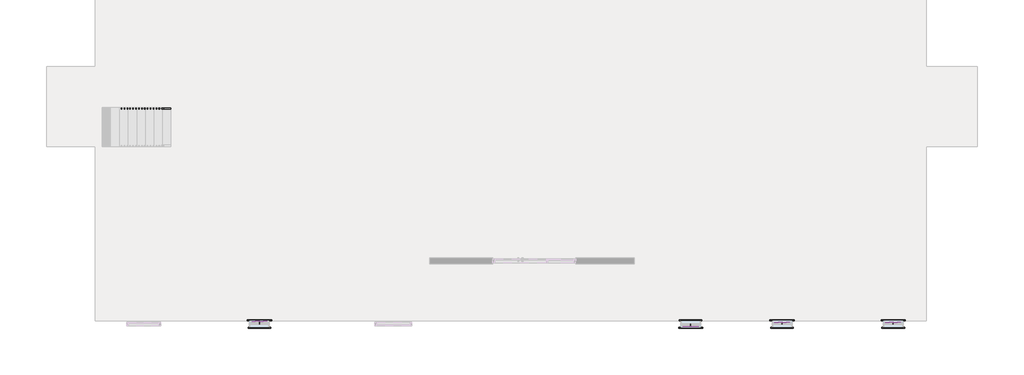
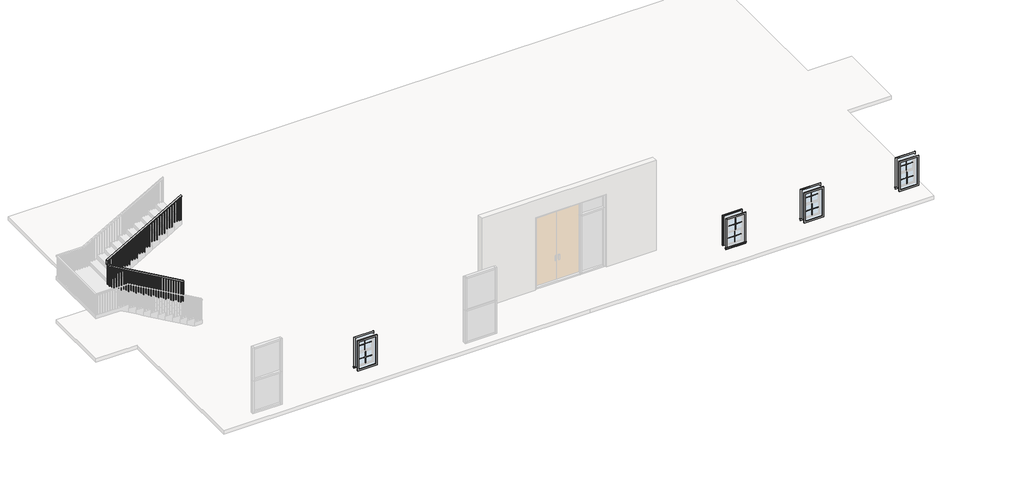
# One storey, part 3 of 3: 16 proxies, 1 railing.
"""IFC4 building model written with IfcOpenShell, lengths in millimetres."""

from ifc_helpers import new_model, si_unit, frame, origin, place, context, project, spatial, polyline, outline, extrude, faceted_brep, transform, mapped, element, save
from components import m_muntin_pattern_2x2_m_muntin_pattern_2x2_8c828626, m_trim_window_exterior_flat_with_sill_7a42a2ef, m_trim_window_interior_flat_picture_frame_c294611c

model = new_model("IFC4")

# Units and contexts
model_context = context("Model", 3, world=origin())
ifc_project = project(units=[si_unit("LENGTHUNIT", "METRE", prefix="MILLI")], contexts=[model_context])

# Site, building, storey
site = spatial("IfcSite", under=ifc_project)
building = spatial("IfcBuilding", under=site)
storey = spatial("IfcBuildingStorey", under=building, Elevation=600.0)

# Proxies
placement = place(None, origin())
m_muntin_pattern_2x2_m_muntin_pattern_2x2_shape = m_muntin_pattern_2x2_m_muntin_pattern_2x2_8c828626(model_context)
element("IfcBuildingElementProxy", 1, Name="M_Muntin Pattern_2x2 : M_Muntin Pattern_2x2", ObjectType="M_Muntin Pattern_2x2 : M_Muntin Pattern_2x2", at=placement, inside=storey, context=model_context, shape_type="MappedRepresentation", body=[
    mapped(m_muntin_pattern_2x2_m_muntin_pattern_2x2_shape, transform((11343.5830368, -12943.1342374, 2136.625), x_axis=(-1.0, 0.0, 0.0), y_axis=(0.0, -1.0, 0.0), z_axis=(0.0, 0.0, 1.0))),
])
element("IfcBuildingElementProxy", 2, Name="M_Muntin Pattern_2x2 : M_Muntin Pattern_2x2", ObjectType="M_Muntin Pattern_2x2 : M_Muntin Pattern_2x2", at=placement, inside=storey, context=model_context, shape_type="MappedRepresentation", body=[
    mapped(m_muntin_pattern_2x2_m_muntin_pattern_2x2_shape, transform((11343.5830368, -12898.6842374, 1590.6), x_axis=(-1.0, 0.0, 0.0), y_axis=(0.0, -1.0, 0.0), z_axis=(0.0, 0.0, 1.0))),
])
element("IfcBuildingElementProxy", 3, Name="M_Muntin Pattern_2x2 : M_Muntin Pattern_2x2", ObjectType="M_Muntin Pattern_2x2 : M_Muntin Pattern_2x2", at=placement, inside=storey, context=model_context, shape_type="MappedRepresentation", body=[
    mapped(m_muntin_pattern_2x2_m_muntin_pattern_2x2_shape, transform((14543.5830368, -12787.9842374, 2136.625), x_axis=(1.0, 0.0, 0.0), y_axis=(0.0, 1.0, 0.0), z_axis=(0.0, 0.0, 1.0))),
])
element("IfcBuildingElementProxy", 4, Name="M_Muntin Pattern_2x2 : M_Muntin Pattern_2x2", ObjectType="M_Muntin Pattern_2x2 : M_Muntin Pattern_2x2", at=placement, inside=storey, context=model_context, shape_type="MappedRepresentation", body=[
    mapped(m_muntin_pattern_2x2_m_muntin_pattern_2x2_shape, transform((14543.5830368, -12832.4342374, 1590.6), x_axis=(1.0, 0.0, 0.0), y_axis=(0.0, 1.0, 0.0), z_axis=(0.0, 0.0, 1.0))),
])
element("IfcBuildingElementProxy", 5, Name="M_Muntin Pattern_2x2 : M_Muntin Pattern_2x2", ObjectType="M_Muntin Pattern_2x2 : M_Muntin Pattern_2x2", at=placement, inside=storey, context=model_context, shape_type="MappedRepresentation", body=[
    mapped(m_muntin_pattern_2x2_m_muntin_pattern_2x2_shape, transform((18431.0830368, -12787.9842374, 2136.625), x_axis=(1.0, 0.0, 0.0), y_axis=(0.0, 1.0, 0.0), z_axis=(0.0, 0.0, 1.0))),
])
element("IfcBuildingElementProxy", 6, Name="M_Muntin Pattern_2x2 : M_Muntin Pattern_2x2", ObjectType="M_Muntin Pattern_2x2 : M_Muntin Pattern_2x2", at=placement, inside=storey, context=model_context, shape_type="MappedRepresentation", body=[
    mapped(m_muntin_pattern_2x2_m_muntin_pattern_2x2_shape, transform((18431.0830368, -12832.4342374, 1590.6), x_axis=(1.0, 0.0, 0.0), y_axis=(0.0, 1.0, 0.0), z_axis=(0.0, 0.0, 1.0))),
])
element("IfcBuildingElementProxy", 7, Name="M_Muntin Pattern_2x2 : M_Muntin Pattern_2x2", ObjectType="M_Muntin Pattern_2x2 : M_Muntin Pattern_2x2", at=placement, inside=storey, context=model_context, shape_type="MappedRepresentation", body=[
    mapped(m_muntin_pattern_2x2_m_muntin_pattern_2x2_shape, transform((-3743.9169632, -12787.9842374, 2136.625), x_axis=(1.0, 0.0, 0.0), y_axis=(0.0, 1.0, 0.0), z_axis=(0.0, 0.0, 1.0))),
])
element("IfcBuildingElementProxy", 8, Name="M_Muntin Pattern_2x2 : M_Muntin Pattern_2x2", ObjectType="M_Muntin Pattern_2x2 : M_Muntin Pattern_2x2", at=placement, inside=storey, context=model_context, shape_type="MappedRepresentation", body=[
    mapped(m_muntin_pattern_2x2_m_muntin_pattern_2x2_shape, transform((-3743.9169632, -12832.4342374, 1590.6), x_axis=(1.0, 0.0, 0.0), y_axis=(0.0, 1.0, 0.0), z_axis=(0.0, 0.0, 1.0))),
])
m_trim_window_exterior_flat_with_sill_shape = m_trim_window_exterior_flat_with_sill_7a42a2ef(model_context)
element("IfcBuildingElementProxy", 9, Name="M_Trim-Window-Exterior-Flat : with Sill", ObjectType="M_Trim-Window-Exterior-Flat : with Sill", at=placement, inside=storey, context=model_context, shape_type="MappedRepresentation", body=[
    mapped(m_trim_window_exterior_flat_with_sill_shape, transform((11343.5830368, -12978.0592374, 2714.4), x_axis=(1.0, 0.0, 0.0), y_axis=(0.0, 0.0, 1.0), z_axis=(0.0, -1.0, 0.0))),
])
element("IfcBuildingElementProxy", 10, Name="M_Trim-Window-Exterior-Flat : with Sill", ObjectType="M_Trim-Window-Exterior-Flat : with Sill", at=placement, inside=storey, context=model_context, shape_type="MappedRepresentation", body=[
    mapped(m_trim_window_exterior_flat_with_sill_shape, transform((14543.5830368, -12753.0592374, 2714.4), x_axis=(-1.0, 0.0, 0.0), y_axis=(0.0, 0.0, 1.0), z_axis=(0.0, 1.0, 0.0))),
])
element("IfcBuildingElementProxy", 11, Name="M_Trim-Window-Exterior-Flat : with Sill", ObjectType="M_Trim-Window-Exterior-Flat : with Sill", at=placement, inside=storey, context=model_context, shape_type="MappedRepresentation", body=[
    mapped(m_trim_window_exterior_flat_with_sill_shape, transform((18431.0830368, -12753.0592374, 2714.4), x_axis=(-1.0, 0.0, 0.0), y_axis=(0.0, 0.0, 1.0), z_axis=(0.0, 1.0, 0.0))),
])
element("IfcBuildingElementProxy", 12, Name="M_Trim-Window-Exterior-Flat : with Sill", ObjectType="M_Trim-Window-Exterior-Flat : with Sill", at=placement, inside=storey, context=model_context, shape_type="MappedRepresentation", body=[
    mapped(m_trim_window_exterior_flat_with_sill_shape, transform((-3743.9169632, -12753.0592374, 2714.4), x_axis=(-1.0, 0.0, 0.0), y_axis=(0.0, 0.0, 1.0), z_axis=(0.0, 1.0, 0.0))),
])
m_trim_window_interior_flat_picture_frame_shape = m_trim_window_interior_flat_picture_frame_c294611c(model_context)
element("IfcBuildingElementProxy", 13, Name="M_Trim-Window-Interior-Flat : Picture Frame", ObjectType="M_Trim-Window-Interior-Flat : Picture Frame", at=placement, inside=storey, context=model_context, shape_type="MappedRepresentation", body=[
    mapped(m_trim_window_interior_flat_picture_frame_shape, transform((11343.5830368, -12753.0592374, 2714.4), x_axis=(-1.0, 0.0, 0.0), y_axis=(0.0, 0.0, 1.0), z_axis=(0.0, 1.0, 0.0))),
])
element("IfcBuildingElementProxy", 14, Name="M_Trim-Window-Interior-Flat : Picture Frame", ObjectType="M_Trim-Window-Interior-Flat : Picture Frame", at=placement, inside=storey, context=model_context, shape_type="MappedRepresentation", body=[
    mapped(m_trim_window_interior_flat_picture_frame_shape, transform((14543.5830368, -12978.0592374, 2714.4), x_axis=(1.0, 0.0, 0.0), y_axis=(0.0, 0.0, 1.0), z_axis=(0.0, -1.0, 0.0))),
])
element("IfcBuildingElementProxy", 15, Name="M_Trim-Window-Interior-Flat : Picture Frame", ObjectType="M_Trim-Window-Interior-Flat : Picture Frame", at=placement, inside=storey, context=model_context, shape_type="MappedRepresentation", body=[
    mapped(m_trim_window_interior_flat_picture_frame_shape, transform((18431.0830368, -12978.0592374, 2714.4), x_axis=(1.0, 0.0, 0.0), y_axis=(0.0, 0.0, 1.0), z_axis=(0.0, -1.0, 0.0))),
])
element("IfcBuildingElementProxy", 16, Name="M_Trim-Window-Interior-Flat : Picture Frame", ObjectType="M_Trim-Window-Interior-Flat : Picture Frame", at=placement, inside=storey, context=model_context, shape_type="MappedRepresentation", body=[
    mapped(m_trim_window_interior_flat_picture_frame_shape, transform((-3743.9169632, -12978.0592374, 2714.4), x_axis=(1.0, 0.0, 0.0), y_axis=(0.0, 0.0, 1.0), z_axis=(0.0, -1.0, 0.0))),
])

# Railing
element("IfcRailing", 17, ObjectType="Handrail - Rectangular", at=placement, inside=storey, context=model_context, shape_type="SolidModel", body=[
    faceted_brep([(-6843.9169632, -5340.9592374, 1671.4285714), (-6843.9169632, -5340.9592374, 1613.8410161), (-6843.9169632, -5290.9592374, 1613.8410161), (-6843.9169632, -5290.9592374, 1671.4285714), (-9769.3169632, -5340.9592374, 3343.0857143), (-9819.3169632, -5340.9592374, 3314.0695875), (-9819.3169632, -5290.9592374, 3314.0695875), (-9769.3169632, -5290.9592374, 3343.0857143), (-9769.3169632, -5340.9592374, 3385.7142857), (-9819.3169632, -5340.9592374, 3335.7142857), (-9819.3169632, -5290.9592374, 3335.7142857), (-9769.3169632, -5290.9592374, 3385.7142857), (-9894.3169632, -5340.9592374, 3385.7142857), (-9894.3169632, -5340.9592374, 3335.7142857), (-9844.3169632, -5290.9592374, 3335.7142857), (-9844.3169632, -5290.9592374, 3385.7142857), (-9894.3169632, -5215.9592374, 3385.7142857), (-9894.3169632, -5215.9592374, 3335.7142857), (-9844.3169632, -5215.9592374, 3335.7142857), (-9844.3169632, -5215.9592374, 3385.7142857), (-9894.3169632, -5190.1592374, 3385.7142857), (-9844.3169632, -5190.1592374, 3385.7142857), (-9844.3169632, -5140.1592374, 3335.7142857), (-9894.3169632, -5140.1592374, 3335.7142857)], [[[0, 1, 2, 3]], [[1, 0, 4, 5]], [[2, 1, 5, 6]], [[3, 2, 6, 7]], [[0, 3, 7, 4]], [[5, 4, 8, 9]], [[6, 5, 9, 10]], [[7, 6, 10, 11]], [[4, 7, 11, 8]], [[9, 8, 12, 13]], [[10, 9, 13, 14]], [[11, 10, 14, 15]], [[8, 11, 15, 12]], [[13, 12, 16, 17]], [[14, 13, 17, 18]], [[15, 14, 18, 19]], [[12, 15, 19, 16]], [[20, 21, 22, 23]], [[17, 16, 20, 23]], [[18, 17, 23, 22]], [[19, 18, 22, 21]], [[16, 19, 21, 20]]]),
    faceted_brep([(-9894.3169632, -5190.1592374, 3385.7142857), (-9894.3169632, -5140.1592374, 3335.7142857), (-9844.3169632, -5140.1592374, 3335.7142857), (-9844.3169632, -5190.1592374, 3385.7142857), (-9894.3169632, -5190.1592374, 3528.3428571), (-9844.3169632, -5190.1592374, 3499.3267304), (-9844.3169632, -5140.1592374, 3499.3267304), (-9894.3169632, -5140.1592374, 3528.3428571)], [[[0, 1, 2, 3]], [[4, 5, 6, 7]], [[1, 0, 4, 7]], [[2, 1, 7, 6]], [[3, 2, 6, 5]], [[0, 3, 5, 4]]]),
    faceted_brep([(-9894.3169632, -5140.1592374, 3528.3428571), (-9844.3169632, -5140.1592374, 3499.3267304), (-9844.3169632, -5190.1592374, 3499.3267304), (-9894.3169632, -5190.1592374, 3528.3428571), (-6843.9169632, -5140.1592374, 5271.4285714), (-6843.9169632, -5190.1592374, 5271.4285714), (-6843.9169632, -5190.1592374, 5213.8410161), (-6843.9169632, -5140.1592374, 5213.8410161)], [[[0, 1, 2, 3]], [[4, 5, 6, 7]], [[1, 0, 4, 7]], [[2, 1, 7, 6]], [[3, 2, 6, 5]], [[0, 3, 5, 4]]]),
    extrude(outline(polyline([(5162.9838732, -6932.9169632), (4200.0, -6932.9169632), (4200.0, -6912.9169632), (5174.4124447, -6912.9169632), (5162.9838732, -6932.9169632)])), frame((0.0, -5175.1592374, 0.0), z_axis=(0.0, 1.0, 0.0), x_axis=(0.0, 0.0, 1.0)), (0.0, 0.0, 1.0), 20.0),
    extrude(outline(polyline([(5104.9267304, -7034.5169632), (4200.0, -7034.5169632), (4200.0, -7014.5169632), (5116.3553018, -7014.5169632), (5104.9267304, -7034.5169632)])), frame((0.0, -5175.1592374, 0.0), z_axis=(0.0, 1.0, 0.0), x_axis=(0.0, 0.0, 1.0)), (0.0, 0.0, 1.0), 20.0),
    extrude(outline(polyline([(5046.8695875, -7136.1169632), (4200.0, -7136.1169632), (4200.0, -7116.1169632), (5058.2981589, -7116.1169632), (5046.8695875, -7136.1169632)])), frame((0.0, -5175.1592374, 0.0), z_axis=(0.0, 1.0, 0.0), x_axis=(0.0, 0.0, 1.0)), (0.0, 0.0, 1.0), 20.0),
    extrude(outline(polyline([(4988.8124447, -7237.7169632), (4028.5714286, -7237.7169632), (4028.5714286, -7217.7169632), (5000.2410161, -7217.7169632), (4988.8124447, -7237.7169632)])), frame((0.0, -5175.1592374, 0.0), z_axis=(0.0, 1.0, 0.0), x_axis=(0.0, 0.0, 1.0)), (0.0, 0.0, 1.0), 20.0),
    extrude(outline(polyline([(4930.7553018, -7339.3169632), (4028.5714286, -7339.3169632), (4028.5714286, -7319.3169632), (4942.1838732, -7319.3169632), (4930.7553018, -7339.3169632)])), frame((0.0, -5175.1592374, 0.0), z_axis=(0.0, 1.0, 0.0), x_axis=(0.0, 0.0, 1.0)), (0.0, 0.0, 1.0), 20.0),
    extrude(outline(polyline([(4872.6981589, -7440.9169632), (4028.5714286, -7440.9169632), (4028.5714286, -7420.9169632), (4884.1267304, -7420.9169632), (4872.6981589, -7440.9169632)])), frame((0.0, -5175.1592374, 0.0), z_axis=(0.0, 1.0, 0.0), x_axis=(0.0, 0.0, 1.0)), (0.0, 0.0, 1.0), 20.0),
    extrude(outline(polyline([(4814.6410161, -7542.5169632), (3857.1428571, -7542.5169632), (3857.1428571, -7522.5169632), (4826.0695875, -7522.5169632), (4814.6410161, -7542.5169632)])), frame((0.0, -5175.1592374, 0.0), z_axis=(0.0, 1.0, 0.0), x_axis=(0.0, 0.0, 1.0)), (0.0, 0.0, 1.0), 20.0),
    extrude(outline(polyline([(4756.5838732, -7644.1169632), (3857.1428571, -7644.1169632), (3857.1428571, -7624.1169632), (4768.0124447, -7624.1169632), (4756.5838732, -7644.1169632)])), frame((0.0, -5175.1592374, 0.0), z_axis=(0.0, 1.0, 0.0), x_axis=(0.0, 0.0, 1.0)), (0.0, 0.0, 1.0), 20.0),
    extrude(outline(polyline([(4698.5267304, -7745.7169632), (3857.1428571, -7745.7169632), (3857.1428571, -7725.7169632), (4709.9553018, -7725.7169632), (4698.5267304, -7745.7169632)])), frame((0.0, -5175.1592374, 0.0), z_axis=(0.0, 1.0, 0.0), x_axis=(0.0, 0.0, 1.0)), (0.0, 0.0, 1.0), 20.0),
    extrude(outline(polyline([(4640.4695875, -7847.3169632), (3685.7142857, -7847.3169632), (3685.7142857, -7827.3169632), (4651.8981589, -7827.3169632), (4640.4695875, -7847.3169632)])), frame((0.0, -5175.1592374, 0.0), z_axis=(0.0, 1.0, 0.0), x_axis=(0.0, 0.0, 1.0)), (0.0, 0.0, 1.0), 20.0),
    extrude(outline(polyline([(4582.4124447, -7948.9169632), (3685.7142857, -7948.9169632), (3685.7142857, -7928.9169632), (4593.8410161, -7928.9169632), (4582.4124447, -7948.9169632)])), frame((0.0, -5175.1592374, 0.0), z_axis=(0.0, 1.0, 0.0), x_axis=(0.0, 0.0, 1.0)), (0.0, 0.0, 1.0), 20.0),
    extrude(outline(polyline([(4524.3553018, -8050.5169632), (3685.7142857, -8050.5169632), (3685.7142857, -8030.5169632), (4535.7838732, -8030.5169632), (4524.3553018, -8050.5169632)])), frame((0.0, -5175.1592374, 0.0), z_axis=(0.0, 1.0, 0.0), x_axis=(0.0, 0.0, 1.0)), (0.0, 0.0, 1.0), 20.0),
    extrude(outline(polyline([(4466.2981589, -8152.1169632), (3514.2857143, -8152.1169632), (3514.2857143, -8132.1169632), (4477.7267304, -8132.1169632), (4466.2981589, -8152.1169632)])), frame((0.0, -5175.1592374, 0.0), z_axis=(0.0, 1.0, 0.0), x_axis=(0.0, 0.0, 1.0)), (0.0, 0.0, 1.0), 20.0),
    extrude(outline(polyline([(4408.2410161, -8253.7169632), (3514.2857143, -8253.7169632), (3514.2857143, -8233.7169632), (4419.6695875, -8233.7169632), (4408.2410161, -8253.7169632)])), frame((0.0, -5175.1592374, 0.0), z_axis=(0.0, 1.0, 0.0), x_axis=(0.0, 0.0, 1.0)), (0.0, 0.0, 1.0), 20.0),
    extrude(outline(polyline([(4350.1838732, -8355.3169632), (3342.8571429, -8355.3169632), (3342.8571429, -8335.3169632), (4361.6124447, -8335.3169632), (4350.1838732, -8355.3169632)])), frame((0.0, -5175.1592374, 0.0), z_axis=(0.0, 1.0, 0.0), x_axis=(0.0, 0.0, 1.0)), (0.0, 0.0, 1.0), 20.0),
    extrude(outline(polyline([(4292.1267304, -8456.9169632), (3342.8571429, -8456.9169632), (3342.8571429, -8436.9169632), (4303.5553018, -8436.9169632), (4292.1267304, -8456.9169632)])), frame((0.0, -5175.1592374, 0.0), z_axis=(0.0, 1.0, 0.0), x_axis=(0.0, 0.0, 1.0)), (0.0, 0.0, 1.0), 20.0),
    extrude(outline(polyline([(4234.0695875, -8558.5169632), (3342.8571429, -8558.5169632), (3342.8571429, -8538.5169632), (4245.4981589, -8538.5169632), (4234.0695875, -8558.5169632)])), frame((0.0, -5175.1592374, 0.0), z_axis=(0.0, 1.0, 0.0), x_axis=(0.0, 0.0, 1.0)), (0.0, 0.0, 1.0), 20.0),
    extrude(outline(polyline([(4176.0124447, -8660.1169632), (3171.4285714, -8660.1169632), (3171.4285714, -8640.1169632), (4187.4410161, -8640.1169632), (4176.0124447, -8660.1169632)])), frame((0.0, -5175.1592374, 0.0), z_axis=(0.0, 1.0, 0.0), x_axis=(0.0, 0.0, 1.0)), (0.0, 0.0, 1.0), 20.0),
    extrude(outline(polyline([(4117.9553018, -8761.7169632), (3171.4285714, -8761.7169632), (3171.4285714, -8741.7169632), (4129.3838732, -8741.7169632), (4117.9553018, -8761.7169632)])), frame((0.0, -5175.1592374, 0.0), z_axis=(0.0, 1.0, 0.0), x_axis=(0.0, 0.0, 1.0)), (0.0, 0.0, 1.0), 20.0),
    extrude(outline(polyline([(4059.8981589, -8863.3169632), (3171.4285714, -8863.3169632), (3171.4285714, -8843.3169632), (4071.3267304, -8843.3169632), (4059.8981589, -8863.3169632)])), frame((0.0, -5175.1592374, 0.0), z_axis=(0.0, 1.0, 0.0), x_axis=(0.0, 0.0, 1.0)), (0.0, 0.0, 1.0), 20.0),
    extrude(outline(polyline([(4001.8410161, -8964.9169632), (3000.0, -8964.9169632), (3000.0, -8944.9169632), (4013.2695875, -8944.9169632), (4001.8410161, -8964.9169632)])), frame((0.0, -5175.1592374, 0.0), z_axis=(0.0, 1.0, 0.0), x_axis=(0.0, 0.0, 1.0)), (0.0, 0.0, 1.0), 20.0),
    extrude(outline(polyline([(3943.7838732, -9066.5169632), (3000.0, -9066.5169632), (3000.0, -9046.5169632), (3955.2124447, -9046.5169632), (3943.7838732, -9066.5169632)])), frame((0.0, -5175.1592374, 0.0), z_axis=(0.0, 1.0, 0.0), x_axis=(0.0, 0.0, 1.0)), (0.0, 0.0, 1.0), 20.0),
    extrude(outline(polyline([(3885.7267304, -9168.1169632), (3000.0, -9168.1169632), (3000.0, -9148.1169632), (3897.1553018, -9148.1169632), (3885.7267304, -9168.1169632)])), frame((0.0, -5175.1592374, 0.0), z_axis=(0.0, 1.0, 0.0), x_axis=(0.0, 0.0, 1.0)), (0.0, 0.0, 1.0), 20.0),
    extrude(outline(polyline([(3827.6695875, -9269.7169632), (2828.5714286, -9269.7169632), (2828.5714286, -9249.7169632), (3839.0981589, -9249.7169632), (3827.6695875, -9269.7169632)])), frame((0.0, -5175.1592374, 0.0), z_axis=(0.0, 1.0, 0.0), x_axis=(0.0, 0.0, 1.0)), (0.0, 0.0, 1.0), 20.0),
    extrude(outline(polyline([(3769.6124447, -9371.3169632), (2828.5714286, -9371.3169632), (2828.5714286, -9351.3169632), (3781.0410161, -9351.3169632), (3769.6124447, -9371.3169632)])), frame((0.0, -5175.1592374, 0.0), z_axis=(0.0, 1.0, 0.0), x_axis=(0.0, 0.0, 1.0)), (0.0, 0.0, 1.0), 20.0),
    extrude(outline(polyline([(3711.5553018, -9472.9169632), (2828.5714286, -9472.9169632), (2828.5714286, -9452.9169632), (3722.9838732, -9452.9169632), (3711.5553018, -9472.9169632)])), frame((0.0, -5175.1592374, 0.0), z_axis=(0.0, 1.0, 0.0), x_axis=(0.0, 0.0, 1.0)), (0.0, 0.0, 1.0), 20.0),
    extrude(outline(polyline([(3653.4981589, -9574.5169632), (2657.1428571, -9574.5169632), (2657.1428571, -9554.5169632), (3664.9267304, -9554.5169632), (3653.4981589, -9574.5169632)])), frame((0.0, -5175.1592374, 0.0), z_axis=(0.0, 1.0, 0.0), x_axis=(0.0, 0.0, 1.0)), (0.0, 0.0, 1.0), 20.0),
    extrude(outline(polyline([(3595.4410161, -9676.1169632), (2657.1428571, -9676.1169632), (2657.1428571, -9656.1169632), (3606.8695875, -9656.1169632), (3595.4410161, -9676.1169632)])), frame((0.0, -5175.1592374, 0.0), z_axis=(0.0, 1.0, 0.0), x_axis=(0.0, 0.0, 1.0)), (0.0, 0.0, 1.0), 20.0),
    extrude(outline(polyline([(3537.3838732, -9777.7169632), (2657.1428571, -9777.7169632), (2657.1428571, -9757.7169632), (3548.8124447, -9757.7169632), (3537.3838732, -9777.7169632)])), frame((0.0, -5175.1592374, 0.0), z_axis=(0.0, 1.0, 0.0), x_axis=(0.0, 0.0, 1.0)), (0.0, 0.0, 1.0), 20.0),
    extrude(outline(polyline([(-9859.3169632, -5224.3592374), (-9879.3169632, -5224.3592374), (-9879.3169632, -5204.3592374), (-9859.3169632, -5204.3592374), (-9859.3169632, -5224.3592374)])), frame((0.0, 0.0, 2485.7142857), z_axis=(0.0, 0.0, 1.0), x_axis=(1.0, 0.0, 0.0)), (0.0, 0.0, 1.0), 850.0),
    extrude(outline(polyline([(-9780.3169632, -5305.9592374), (-9780.3169632, -5325.9592374), (-9800.3169632, -5325.9592374), (-9800.3169632, -5305.9592374), (-9780.3169632, -5305.9592374)])), frame((0.0, 0.0, 2314.2857143), z_axis=(0.0, 0.0, 1.0), x_axis=(1.0, 0.0, 0.0)), (0.0, 0.0, 1.0), 1021.4285714),
    extrude(outline(polyline([(2314.2857143, -9678.7169632), (3233.7267304, -9678.7169632), (3245.1553018, -9698.7169632), (2314.2857143, -9698.7169632), (2314.2857143, -9678.7169632)])), frame((0.0, -5325.9592374, 0.0), z_axis=(0.0, 1.0, 0.0), x_axis=(0.0, 0.0, 1.0)), (0.0, 0.0, 1.0), 20.0),
    extrude(outline(polyline([(2314.2857143, -9577.1169632), (3175.6695875, -9577.1169632), (3187.0981589, -9597.1169632), (2314.2857143, -9597.1169632), (2314.2857143, -9577.1169632)])), frame((0.0, -5325.9592374, 0.0), z_axis=(0.0, 1.0, 0.0), x_axis=(0.0, 0.0, 1.0)), (0.0, 0.0, 1.0), 20.0),
    extrude(outline(polyline([(2142.8571429, -9475.5169632), (3117.6124447, -9475.5169632), (3129.0410161, -9495.5169632), (2142.8571429, -9495.5169632), (2142.8571429, -9475.5169632)])), frame((0.0, -5325.9592374, 0.0), z_axis=(0.0, 1.0, 0.0), x_axis=(0.0, 0.0, 1.0)), (0.0, 0.0, 1.0), 20.0),
    extrude(outline(polyline([(2142.8571429, -9373.9169632), (3059.5553018, -9373.9169632), (3070.9838732, -9393.9169632), (2142.8571429, -9393.9169632), (2142.8571429, -9373.9169632)])), frame((0.0, -5325.9592374, 0.0), z_axis=(0.0, 1.0, 0.0), x_axis=(0.0, 0.0, 1.0)), (0.0, 0.0, 1.0), 20.0),
    extrude(outline(polyline([(2142.8571429, -9272.3169632), (3001.4981589, -9272.3169632), (3012.9267304, -9292.3169632), (2142.8571429, -9292.3169632), (2142.8571429, -9272.3169632)])), frame((0.0, -5325.9592374, 0.0), z_axis=(0.0, 1.0, 0.0), x_axis=(0.0, 0.0, 1.0)), (0.0, 0.0, 1.0), 20.0),
    extrude(outline(polyline([(1971.4285714, -9170.7169632), (2943.4410161, -9170.7169632), (2954.8695875, -9190.7169632), (1971.4285714, -9190.7169632), (1971.4285714, -9170.7169632)])), frame((0.0, -5325.9592374, 0.0), z_axis=(0.0, 1.0, 0.0), x_axis=(0.0, 0.0, 1.0)), (0.0, 0.0, 1.0), 20.0),
    extrude(outline(polyline([(1971.4285714, -9069.1169632), (2885.3838732, -9069.1169632), (2896.8124447, -9089.1169632), (1971.4285714, -9089.1169632), (1971.4285714, -9069.1169632)])), frame((0.0, -5325.9592374, 0.0), z_axis=(0.0, 1.0, 0.0), x_axis=(0.0, 0.0, 1.0)), (0.0, 0.0, 1.0), 20.0),
    extrude(outline(polyline([(1971.4285714, -8967.5169632), (2827.3267304, -8967.5169632), (2838.7553018, -8987.5169632), (1971.4285714, -8987.5169632), (1971.4285714, -8967.5169632)])), frame((0.0, -5325.9592374, 0.0), z_axis=(0.0, 1.0, 0.0), x_axis=(0.0, 0.0, 1.0)), (0.0, 0.0, 1.0), 20.0),
    extrude(outline(polyline([(1800.0, -8865.9169632), (2769.2695875, -8865.9169632), (2780.6981589, -8885.9169632), (1800.0, -8885.9169632), (1800.0, -8865.9169632)])), frame((0.0, -5325.9592374, 0.0), z_axis=(0.0, 1.0, 0.0), x_axis=(0.0, 0.0, 1.0)), (0.0, 0.0, 1.0), 20.0),
    extrude(outline(polyline([(1800.0, -8764.3169632), (2711.2124447, -8764.3169632), (2722.6410161, -8784.3169632), (1800.0, -8784.3169632), (1800.0, -8764.3169632)])), frame((0.0, -5325.9592374, 0.0), z_axis=(0.0, 1.0, 0.0), x_axis=(0.0, 0.0, 1.0)), (0.0, 0.0, 1.0), 20.0),
    extrude(outline(polyline([(1800.0, -8662.7169632), (2653.1553018, -8662.7169632), (2664.5838732, -8682.7169632), (1800.0, -8682.7169632), (1800.0, -8662.7169632)])), frame((0.0, -5325.9592374, 0.0), z_axis=(0.0, 1.0, 0.0), x_axis=(0.0, 0.0, 1.0)), (0.0, 0.0, 1.0), 20.0),
    extrude(outline(polyline([(1628.5714286, -8561.1169632), (2595.0981589, -8561.1169632), (2606.5267304, -8581.1169632), (1628.5714286, -8581.1169632), (1628.5714286, -8561.1169632)])), frame((0.0, -5325.9592374, 0.0), z_axis=(0.0, 1.0, 0.0), x_axis=(0.0, 0.0, 1.0)), (0.0, 0.0, 1.0), 20.0),
    extrude(outline(polyline([(1628.5714286, -8459.5169632), (2537.0410161, -8459.5169632), (2548.4695875, -8479.5169632), (1628.5714286, -8479.5169632), (1628.5714286, -8459.5169632)])), frame((0.0, -5325.9592374, 0.0), z_axis=(0.0, 1.0, 0.0), x_axis=(0.0, 0.0, 1.0)), (0.0, 0.0, 1.0), 20.0),
    extrude(outline(polyline([(1628.5714286, -8357.9169632), (2478.9838732, -8357.9169632), (2490.4124447, -8377.9169632), (1628.5714286, -8377.9169632), (1628.5714286, -8357.9169632)])), frame((0.0, -5325.9592374, 0.0), z_axis=(0.0, 1.0, 0.0), x_axis=(0.0, 0.0, 1.0)), (0.0, 0.0, 1.0), 20.0),
    extrude(outline(polyline([(1457.1428571, -8256.3169632), (2420.9267304, -8256.3169632), (2432.3553018, -8276.3169632), (1457.1428571, -8276.3169632), (1457.1428571, -8256.3169632)])), frame((0.0, -5325.9592374, 0.0), z_axis=(0.0, 1.0, 0.0), x_axis=(0.0, 0.0, 1.0)), (0.0, 0.0, 1.0), 20.0),
    extrude(outline(polyline([(1457.1428571, -8154.7169632), (2362.8695875, -8154.7169632), (2374.2981589, -8174.7169632), (1457.1428571, -8174.7169632), (1457.1428571, -8154.7169632)])), frame((0.0, -5325.9592374, 0.0), z_axis=(0.0, 1.0, 0.0), x_axis=(0.0, 0.0, 1.0)), (0.0, 0.0, 1.0), 20.0),
    extrude(outline(polyline([(1457.1428571, -8053.1169632), (2304.8124447, -8053.1169632), (2316.2410161, -8073.1169632), (1457.1428571, -8073.1169632), (1457.1428571, -8053.1169632)])), frame((0.0, -5325.9592374, 0.0), z_axis=(0.0, 1.0, 0.0), x_axis=(0.0, 0.0, 1.0)), (0.0, 0.0, 1.0), 20.0),
    extrude(outline(polyline([(1285.7142857, -7951.5169632), (2246.7553018, -7951.5169632), (2258.1838732, -7971.5169632), (1285.7142857, -7971.5169632), (1285.7142857, -7951.5169632)])), frame((0.0, -5325.9592374, 0.0), z_axis=(0.0, 1.0, 0.0), x_axis=(0.0, 0.0, 1.0)), (0.0, 0.0, 1.0), 20.0),
    extrude(outline(polyline([(1285.7142857, -7849.9169632), (2188.6981589, -7849.9169632), (2200.1267304, -7869.9169632), (1285.7142857, -7869.9169632), (1285.7142857, -7849.9169632)])), frame((0.0, -5325.9592374, 0.0), z_axis=(0.0, 1.0, 0.0), x_axis=(0.0, 0.0, 1.0)), (0.0, 0.0, 1.0), 20.0),
    extrude(outline(polyline([(1285.7142857, -7748.3169632), (2130.6410161, -7748.3169632), (2142.0695875, -7768.3169632), (1285.7142857, -7768.3169632), (1285.7142857, -7748.3169632)])), frame((0.0, -5325.9592374, 0.0), z_axis=(0.0, 1.0, 0.0), x_axis=(0.0, 0.0, 1.0)), (0.0, 0.0, 1.0), 20.0),
    extrude(outline(polyline([(1114.2857143, -7646.7169632), (2072.5838732, -7646.7169632), (2084.0124447, -7666.7169632), (1114.2857143, -7666.7169632), (1114.2857143, -7646.7169632)])), frame((0.0, -5325.9592374, 0.0), z_axis=(0.0, 1.0, 0.0), x_axis=(0.0, 0.0, 1.0)), (0.0, 0.0, 1.0), 20.0),
    extrude(outline(polyline([(1114.2857143, -7545.1169632), (2014.5267304, -7545.1169632), (2025.9553018, -7565.1169632), (1114.2857143, -7565.1169632), (1114.2857143, -7545.1169632)])), frame((0.0, -5325.9592374, 0.0), z_axis=(0.0, 1.0, 0.0), x_axis=(0.0, 0.0, 1.0)), (0.0, 0.0, 1.0), 20.0),
    extrude(outline(polyline([(1114.2857143, -7443.5169632), (1956.4124447, -7443.5169632), (1967.8410161, -7463.5169632), (1114.2857143, -7463.5169632), (1114.2857143, -7443.5169632)])), frame((0.0, -5325.9592374, 0.0), z_axis=(0.0, 1.0, 0.0), x_axis=(0.0, 0.0, 1.0)), (0.0, 0.0, 1.0), 20.0),
    extrude(outline(polyline([(942.8571429, -7341.9169632), (1898.4124447, -7341.9169632), (1909.8410161, -7361.9169632), (942.8571429, -7361.9169632), (942.8571429, -7341.9169632)])), frame((0.0, -5325.9592374, 0.0), z_axis=(0.0, 1.0, 0.0), x_axis=(0.0, 0.0, 1.0)), (0.0, 0.0, 1.0), 20.0),
    extrude(outline(polyline([(942.8571429, -7240.3169632), (1840.3553018, -7240.3169632), (1851.7838732, -7260.3169632), (942.8571429, -7260.3169632), (942.8571429, -7240.3169632)])), frame((0.0, -5325.9592374, 0.0), z_axis=(0.0, 1.0, 0.0), x_axis=(0.0, 0.0, 1.0)), (0.0, 0.0, 1.0), 20.0),
    extrude(outline(polyline([(942.8571429, -7138.7169632), (1782.2981589, -7138.7169632), (1793.7267304, -7158.7169632), (942.8571429, -7158.7169632), (942.8571429, -7138.7169632)])), frame((0.0, -5325.9592374, 0.0), z_axis=(0.0, 1.0, 0.0), x_axis=(0.0, 0.0, 1.0)), (0.0, 0.0, 1.0), 20.0),
    extrude(outline(polyline([(771.4285714, -7037.1169632), (1724.2410161, -7037.1169632), (1735.6695875, -7057.1169632), (771.4285714, -7057.1169632), (771.4285714, -7037.1169632)])), frame((0.0, -5325.9592374, 0.0), z_axis=(0.0, 1.0, 0.0), x_axis=(0.0, 0.0, 1.0)), (0.0, 0.0, 1.0), 20.0),
    extrude(outline(polyline([(771.4285714, -6935.5169632), (1666.1838732, -6935.5169632), (1677.6124447, -6955.5169632), (771.4285714, -6955.5169632), (771.4285714, -6935.5169632)])), frame((0.0, -5325.9592374, 0.0), z_axis=(0.0, 1.0, 0.0), x_axis=(0.0, 0.0, 1.0)), (0.0, 0.0, 1.0), 20.0),
    extrude(outline(polyline([(-9859.3169632, -5175.1592374), (-9879.3169632, -5175.1592374), (-9879.3169632, -5155.1592374), (-9859.3169632, -5155.1592374), (-9859.3169632, -5175.1592374)])), frame((0.0, 0.0, 2485.7142857), z_axis=(0.0, 0.0, 1.0), x_axis=(1.0, 0.0, 0.0)), (0.0, 0.0, 1.0), 850.0),
    extrude(outline(polyline([(-9859.3169632, -5305.9592374), (-9859.3169632, -5325.9592374), (-9879.3169632, -5325.9592374), (-9879.3169632, -5305.9592374), (-9859.3169632, -5305.9592374)])), frame((0.0, 0.0, 2485.7142857), z_axis=(0.0, 0.0, 1.0), x_axis=(1.0, 0.0, 0.0)), (0.0, 0.0, 1.0), 850.0),
    extrude(outline(polyline([(5202.6981589, -6863.4169632), (4200.0, -6863.4169632), (4200.0, -6843.4169632), (5214.1267304, -6843.4169632), (5202.6981589, -6863.4169632)])), frame((0.0, -5175.1592374, 0.0), z_axis=(0.0, 1.0, 0.0), x_axis=(0.0, 0.0, 1.0)), (0.0, 0.0, 1.0), 20.0),
    extrude(outline(polyline([(771.4285714, -6843.4169632), (1613.5553018, -6843.4169632), (1624.9838732, -6863.4169632), (771.4285714, -6863.4169632), (771.4285714, -6843.4169632)])), frame((0.0, -5325.9592374, 0.0), z_axis=(0.0, 1.0, 0.0), x_axis=(0.0, 0.0, 1.0)), (0.0, 0.0, 1.0), 20.0),
])

save(model, "model.ifc")

# Revit data of these elements
# Type "M_Muntin Pattern_2x2 : M_Muntin Pattern_2x2"
#   Width [instance default] = 1200 mm
#   Thickness = 12.7 mm
#   Height [instance default] = 1200 mm
#   Distance = 19.05 mm
#   Interior Material [instance default] = none
#   Exterior Material [instance default] = none
#   Default Elevation = 0
# Type "M_Trim-Window-Exterior-Flat : with Sill"
#   Trim Width = 60 mm
#   Trim Thickness_Picture Frame = 30 mm
#   Trim Thickness_with Sill = 19.05 mm
#   Sill Thickness = 30 mm
#   Opening Width [instance default] = 600 mm
#   Opening Height [instance default] = 900 mm
#   Default Elevation = 1200 mm
#   Sill = yes
#   Picture Frame = no
#   Trim Material [instance default] = none
# Type "M_Trim-Window-Interior-Flat : Picture Frame"
#   Trim Thickness_Picture Frame = 30 mm
#   Trim Width = 60 mm
#   Trim Thickness_with Sill = 20 mm
#   Sill Thickness = 30 mm
#   Opening Width [instance default] = 600 mm
#   Opening Height [instance default] = 900 mm
#   Default Elevation = 1200 mm
#   Sill = no
#   Picture Frame = yes
#   Trim Material [instance default] = none
# Type "Handrail - Rectangular"
#   Assembly Code = "C2010400"
#   built-in parameter 1008612 = 0.0416667 (stored number, unit not read)
#   built-in parameter 1008611 = 0.0416667 (stored number, unit not read)
#   built-in parameter 1008609 = 0.333333 (stored number, unit not read)
#   built-in parameter 1008604 = 0.166667 (stored number, unit not read)
#   built-in parameter 1008603 = 0.166667 (stored number, unit not read)
#   Railing Height = 900 mm
#   built-in parameter 1008630 = 2
#   built-in parameter 1008610 = 2
# Elements 1, 2, 3, 4, 5, 6, 7, 8 (IfcBuildingElementProxy, "M_Muntin Pattern_2x2 : M_Muntin Pattern_2x2")
#   Width = 547.6 mm
#   Height = 501.575 mm
#   Interior Material = Wood - Stained
#   Exterior Material = Clad - White
#   Phase Created = New Construction
#   Materials on its faces: "Clad - White", "Wood - Stained"
# Elements 9, 10, 11, 12 (IfcBuildingElementProxy, "M_Trim-Window-Exterior-Flat : with Sill")
#   Opening Width = 700 mm
#   Opening Height = 1200 mm
#   Trim Material = Clad - White
#   Phase Created = New Construction
#   Materials on its faces: "Clad - White"
# Elements 13, 14, 15, 16 (IfcBuildingElementProxy, "M_Trim-Window-Interior-Flat : Picture Frame")
#   Opening Width = 700 mm
#   Opening Height = 1200 mm
#   Trim Material = Wood - Stained
#   Phase Created = New Construction
#   Materials on its faces: "Wood - Stained"
# Element 17 (IfcRailing, "Handrail - Rectangular")
#   Phase Created = New Construction
# Materials
#   "Clad - White": class "Wood", colour RGB 245 245 243, transparency 0, Cost = 0
#   "Wood - Stained": class "Wood", colour RGB 173 132 96, transparency 0, Cost = 0
